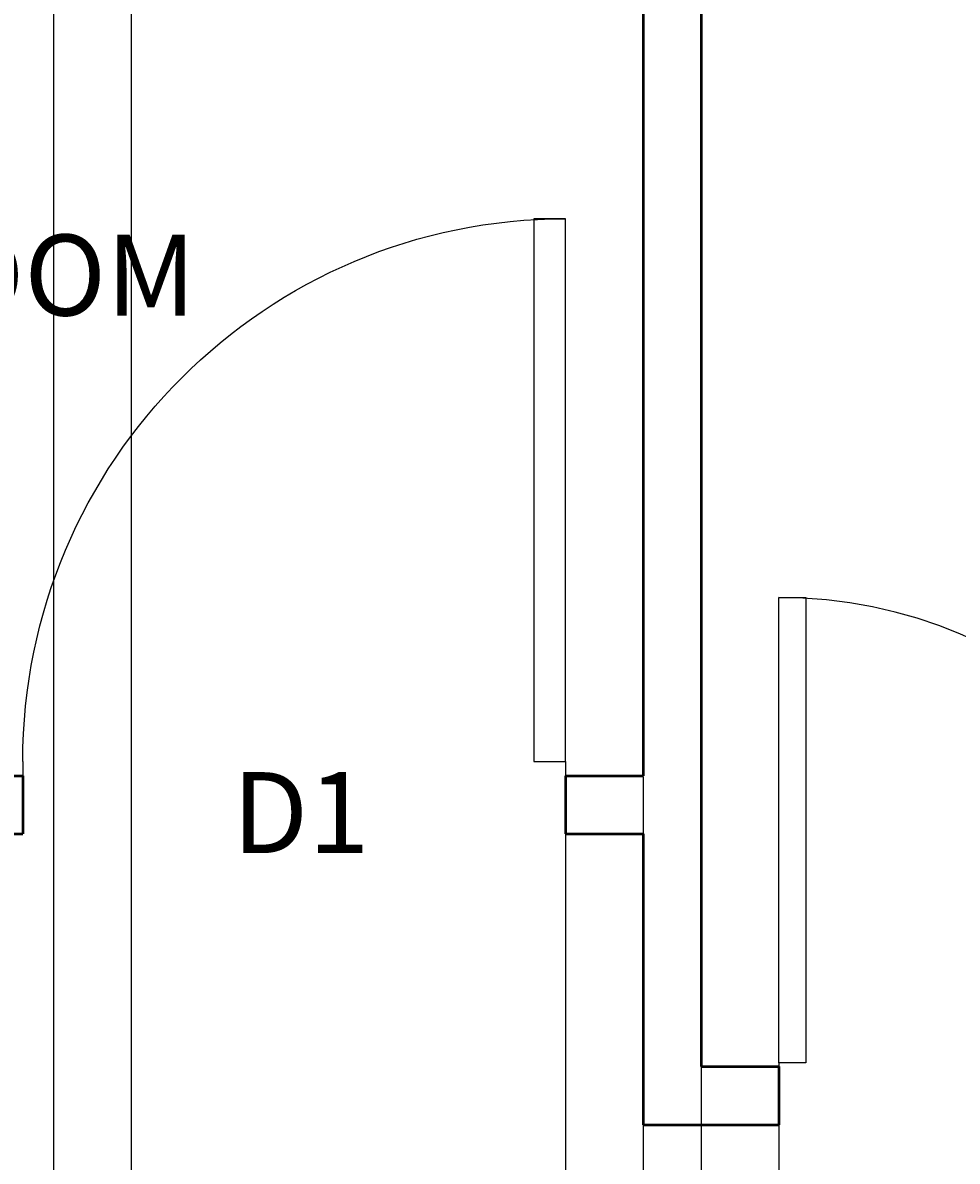
# Model space of a CAD drawing. Units: inches. Extents: x 7359 to 7979, y 33027 to 34263.
# Tile 15 of 32: x 7691 to 7764, y 33446 to 33534. Entities that reach past the tile are written whole.
import ezdxf

# ---------------------------------------------------------------- set-up
doc = ezdxf.new("R2010")
doc.units = ezdxf.units.IN
for name, color, linetype, lineweight in [('A-ANNO-DIMS', 2, 'Continuous', 18), ('A-ANNO-TEXT', 3, 'Continuous', 18), ('A-AREA-IDEN', 7, 'Continuous', 18), ('A-DOOR', 3, 'Continuous', 25), ('A-WALL', 7, 'Continuous', 50)]:
    doc.layers.add(name, color=color, linetype=linetype, lineweight=lineweight)
doc.styles.get("Standard").update_dxf_attribs({"font": 'arial.ttf'})
doc.dimstyles.get("Standard").update_dxf_attribs({"dimtxt": 0.18, "dimasz": 0.18, "dimexe": 0.18, "dimexo": 0.0625, "dimgap": 0.09, "dimtad": 0, "dimtih": 1, "dimtoh": 1, "dimdec": 4, "dimzin": 0, "dimdsep": 46, "dimtxsty": 'Standard', "dimcen": 0.09, "dimadec": 0, "dimazin": 0, "dimtfac": 1, "dimtdec": 4, "dimtofl": 0, "dimtmove": 0, "dimatfit": 3, "dimfxl": 1, "dimtolj": 1, "dimtzin": 0, "dimarcsym": 0})

# ---------------------------------------------------------------- blocks, each defined once
blk = doc.blocks.new('*U2')
for p, q in [((0, 0), (0, -100)), ((750, 0), (750, -100))]:
    blk.add_line(p, q)
blk.add_lwpolyline([(0, 0), (0, 750), (43.75, 750), (43.75, 0)], close=True)
blk.add_arc((0, 0), 750, 0, 90)
blk = doc.blocks.new('*D74')
at = {"layer": 'A-ANNO-DIMS', "color": 0, "lineweight": -2, "transparency": 16777216}
for p, q in [((7743.727, 33618.1), (7743.727, 33027.177)), ((7787.034, 33618.1), (7787.034, 33027.177)), ((7743.907, 33027.357), (7765, 33027.357)), ((7786.854, 33027.357), (7765.76, 33027.357))]:
    blk.add_line(p, q, dxfattribs=at)
at = {"layer": 'A-ANNO-DIMS', "color": 0, "transparency": 16777216}
for points in [[(7743.907, 33027.387), (7743.907, 33027.327), (7743.727, 33027.357)], [(7786.854, 33027.387), (7786.854, 33027.327), (7787.034, 33027.357)]]:
    blk.add_solid(points, dxfattribs=at)
at = {"layer": 'Defpoints', "color": 0, "transparency": 16777216}
for p in [(7743.727, 33618.162), (7787.034, 33618.162), (7787.034, 33027.357)]:
    blk.add_point(p, dxfattribs=at)
at = {"layer": 'A-ANNO-DIMS', "color": 0, "transparency": 16777216, "insert": (7765.38, 33027.357), "char_height": 0.18, "attachment_point": 5}
blk.add_mtext('\\A1;43.31', dxfattribs=at)
blk = doc.blocks.new('*D86')
at = {"layer": 'A-ANNO-DIMS', "color": 0, "lineweight": -2, "transparency": 16777216}
for p, q in [((7733.226578, 33475.599789), (7733.226578, 33027.176807)), ((7739.226578, 33475.599789), (7739.226578, 33027.176807)), ((7733.406578, 33027.356807), (7736.077151, 33027.356807)), ((7739.046578, 33027.356807), (7736.376005, 33027.356807))]:
    blk.add_line(p, q, dxfattribs=at)
at = {"layer": 'A-ANNO-DIMS', "color": 0, "transparency": 16777216}
for points in [[(7733.406578, 33027.386807), (7733.406578, 33027.326807), (7733.226578, 33027.356807)], [(7739.046578, 33027.386807), (7739.046578, 33027.326807), (7739.226578, 33027.356807)]]:
    blk.add_solid(points, dxfattribs=at)
at = {"layer": 'Defpoints', "color": 0, "transparency": 16777216}
for p in [(7733.226578, 33475.662289), (7739.226578, 33475.662289), (7739.226578, 33027.356807)]:
    blk.add_point(p, dxfattribs=at)
at = {"layer": 'A-ANNO-DIMS', "color": 0, "transparency": 16777216, "insert": (7736.226578, 33027.356807), "char_height": 0.18, "attachment_point": 5}
blk.add_mtext('\\A1;6', dxfattribs=at)
blk = doc.blocks.new('*D87')
at = {"layer": 'A-ANNO-DIMS', "color": 0, "lineweight": -2, "transparency": 16777216}
for p, q in [((7743.726578, 33453.099789), (7743.726578, 33027.176807)), ((7749.726578, 33453.099789), (7749.726578, 33027.176807)), ((7743.906578, 33027.356807), (7746.577151, 33027.356807)), ((7749.546578, 33027.356807), (7746.876005, 33027.356807))]:
    blk.add_line(p, q, dxfattribs=at)
at = {"layer": 'A-ANNO-DIMS', "color": 0, "transparency": 16777216}
for points in [[(7743.906578, 33027.386807), (7743.906578, 33027.326807), (7743.726578, 33027.356807)], [(7749.546578, 33027.386807), (7749.546578, 33027.326807), (7749.726578, 33027.356807)]]:
    blk.add_solid(points, dxfattribs=at)
at = {"layer": 'Defpoints', "color": 0, "transparency": 16777216}
for p in [(7743.726578, 33453.162289), (7749.726578, 33453.162289), (7749.726578, 33027.356807)]:
    blk.add_point(p, dxfattribs=at)
at = {"layer": 'A-ANNO-DIMS', "color": 0, "transparency": 16777216, "insert": (7746.726578, 33027.356807), "char_height": 0.18, "attachment_point": 5}
blk.add_mtext('\\A1;6', dxfattribs=at)
blk = doc.blocks.new('*D89')
at = {"layer": 'A-ANNO-DIMS', "color": 0, "lineweight": -2, "transparency": 16777216}
for p, q in [((7693.626578, 33301.124789), (7693.626578, 33657.242289)), ((7693.806578, 33657.062289), (7696.477151, 33657.062289)), ((7699.446578, 33657.062289), (7696.776005, 33657.062289)), ((7699.626578, 33301.124789), (7699.626578, 33657.242289))]:
    blk.add_line(p, q, dxfattribs=at)
at = {"layer": 'A-ANNO-DIMS', "color": 0, "transparency": 16777216}
for points in [[(7693.806578, 33657.092289), (7693.806578, 33657.032289), (7693.626578, 33657.062289)], [(7699.446578, 33657.092289), (7699.446578, 33657.032289), (7699.626578, 33657.062289)]]:
    blk.add_solid(points, dxfattribs=at)
at = {"layer": 'Defpoints', "color": 0, "transparency": 16777216}
for p in [(7699.626578, 33657.062289), (7693.626578, 33301.062289), (7699.626578, 33301.062289)]:
    blk.add_point(p, dxfattribs=at)
at = {"layer": 'A-ANNO-DIMS', "color": 0, "transparency": 16777216, "insert": (7696.626578, 33657.062289), "char_height": 0.18, "attachment_point": 5}
blk.add_mtext('\\A1;6', dxfattribs=at)

msp = doc.modelspace()

# ---------------------------------------------------------------- linework, layer by layer
at = {"layer": 'A-WALL'}
for p, q in [((7739.2266, 33618.1623), (7739.2266, 33475.6623)), ((7743.7266, 33618.1623), (7743.7266, 33453.1623)), ((7739.2266, 33488.6623), (7739.2266, 33475.6623)), ((7613.2266, 33475.6623), (7691.2266, 33475.6623)), ((7691.2266, 33475.6623), (7691.2266, 33471.1623)), ((7733.2266, 33475.6623), (7739.2266, 33475.6623)), ((7733.2266, 33475.6623), (7733.2266, 33471.1623)), ((7602.7266, 33471.1623), (7691.2266, 33471.1623)), ((7733.2266, 33471.1623), (7739.2266, 33471.1623)), ((7739.2266, 33471.1623), (7739.2266, 33448.6623)), ((7743.7266, 33453.1623), (7749.7266, 33453.1623)), ((7749.7266, 33453.1623), (7749.7266, 33448.6623)), ((7739.2266, 33448.6623), (7749.7266, 33448.6623))]:
    msp.add_line(p, q, dxfattribs=at)

# ---------------------------------------------------------------- block references
at = {"layer": 'A-DOOR'}
for p, xscale, yscale, zscale in [((7733.2266, 33476.7623), -0.0559999819687567, 0.0559999819687567, 0.0559999819687567), ((7749.7266, 33453.4623), 0.0479999999999996, 0.0479999999999996, 0.0479999999999996)]:
    msp.add_blockref('*U2', p, dxfattribs=dict(at, xscale=xscale, yscale=yscale, zscale=zscale))

# ---------------------------------------------------------------- texts
at = {"layer": 'A-ANNO-TEXT'}
msp.add_text('D1', height=6.25941, dxfattribs=at).set_placement((7707.4372, 33469.6849))
at = {"layer": 'A-AREA-IDEN'}
msp.add_text('CHILDRENS BEDROOM', height=6.259411, dxfattribs=at).set_placement((7614.7656, 33511.2719))

# ---------------------------------------------------------------- dimensions: what is measured, and where the dimension line sits
at = {"layer": 'A-ANNO-DIMS'}
for base, p1, p2, override, picture, middle in [((7699.6266, 33657.0623), (7693.6266, 33301.0623), (7699.6266, 33301.0623), {"dimdec": 0, "dimlfac": 1, "dimrnd": 0, "dimzin": 0, "dimdsep": 46, "dimlunit": 2}, '*D89', (7696.6266, 33657.0623)), ((7787.0342, 33027.3568), (7743.7266, 33618.1623), (7787.0342, 33618.1623), {"dimdec": 2, "dimlfac": 1, "dimrnd": 0, "dimzin": 0, "dimdsep": 46, "dimlunit": 2}, '*D74', (7765.3804, 33027.3568)), ((7739.2266, 33027.3568), (7733.2266, 33475.6623), (7739.2266, 33475.6623), {"dimdec": 0, "dimlfac": 1, "dimrnd": 0, "dimzin": 0, "dimdsep": 46, "dimlunit": 2}, '*D86', (7736.2266, 33027.3568)), ((7749.7266, 33027.3568), (7743.7266, 33453.1623), (7749.7266, 33453.1623), {"dimdec": 0, "dimlfac": 1, "dimrnd": 0, "dimzin": 0, "dimdsep": 46, "dimlunit": 2}, '*D87', (7746.7266, 33027.3568))]:
    dim = msp.add_linear_dim(base=base, p1=p1, p2=p2, dimstyle='Standard', override=override, dxfattribs=at)
    dim.commit()
    dim.dimension.update_dxf_attribs({"geometry": picture, "text_midpoint": middle})

doc.saveas('drawing.dxf')
